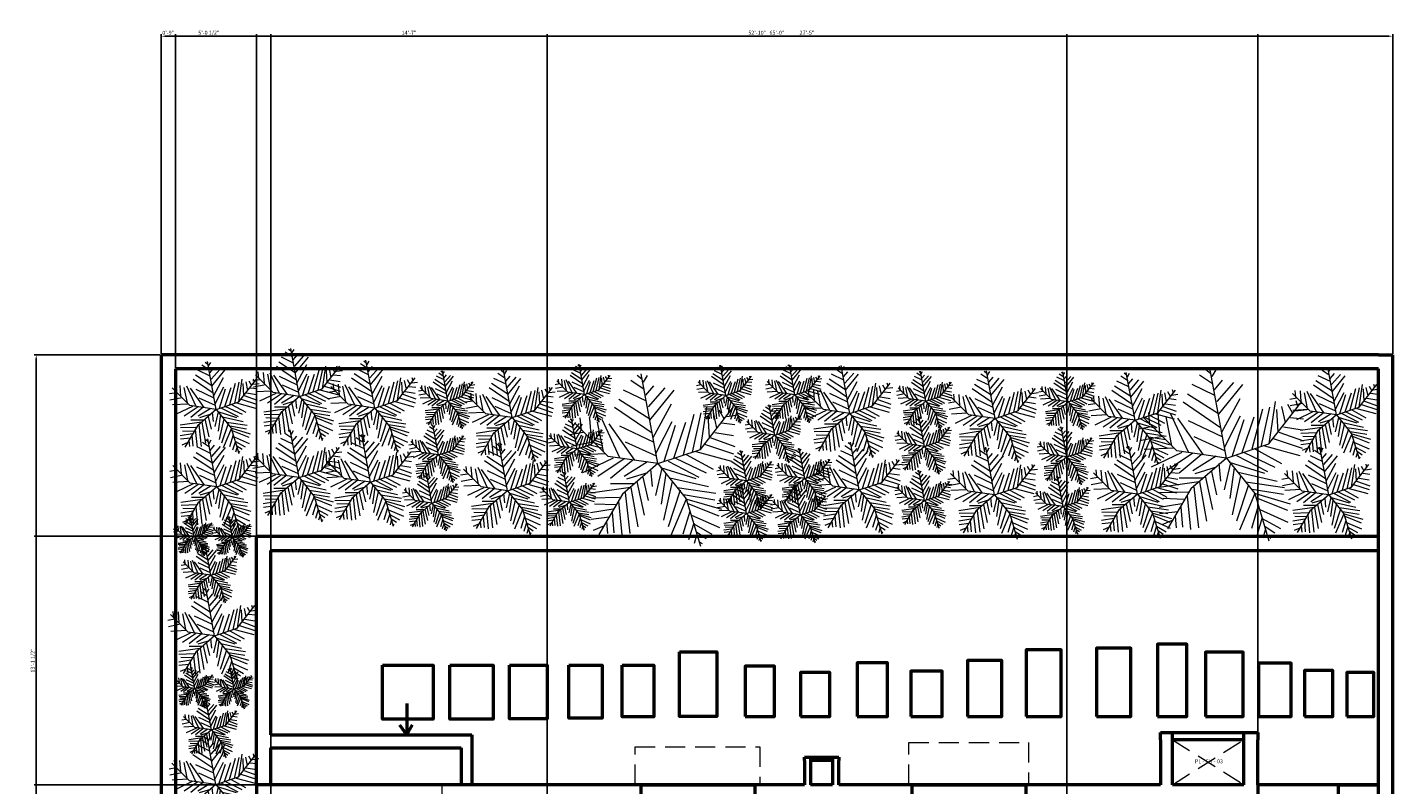
# Model space of a CAD drawing. Units: inches. Extents: x 5312 to 23584, y 2846 to 7447.
# Tile 4 of 12: x 8876 to 9740, y 3738 to 4217. Entities that reach past the tile are written whole.
import ezdxf

# ---------------------------------------------------------------- set-up
doc = ezdxf.new("R2010")
doc.units = ezdxf.units.IN
doc.linetypes.add('DASHED', pattern=[19.05, 12.7, -6.35])
for name, color, linetype, lineweight in [('A-ANNO-DIMS', 2, 'Continuous', 18), ('A-ANNO-TEXT', 3, 'Continuous', 18), ('A-FLOR-OVHD', 8, 'DASHED', 18), ('A-WALL', 7, 'Continuous', 50), ('L-PLNT', 82, 'Continuous', 13)]:
    doc.layers.add(name, color=color, linetype=linetype, lineweight=lineweight)
doc.styles.get("Standard").update_dxf_attribs({"font": 'arial.ttf'})
doc.dimstyles.new('ISO-25', dxfattribs={"dimtxt": 2.5, "dimasz": 2.5, "dimexe": 1.25, "dimexo": 0.625, "dimtad": 1, "dimlunit": 3, "dimtxsty": 'Standard', "dimcen": 2.5, "dimadec": 0, "dimazin": 0, "dimtfac": 1, "dimtmove": 0, "dimatfit": 3, "dimfxl": 1, "dimarcsym": 0})

# ---------------------------------------------------------------- blocks, each defined once
blk = doc.blocks.new('*U18')
for p, q in [((-8.737, 47.138), (-17.069, 52.711)), ((-10.186, 53.64), (-13.084, 55.962)), ((0, 0), (-10.5, 57)), ((-9.099, 51.782), (-6.563, 55.962)), ((-7.288, 39.707), (-21.778, 46.673)), ((-7.65, 43.423), (-2.578, 49.46)), ((-5.839, 35.992), (4.667, 48.067)), ((-5.114, 27.632), (10.463, 46.673)), ((-3.665, 19.273), (-27.574, 35.527)), ((-5.114, 28.097), (-24.676, 40.636)), ((-2.941, 16.486), (8.652, 37.85)), ((27, 9), (48, 36)), ((27.127, 9.056), (31.112, 35.992)), ((44.153, 36.456), (45.239, 32.741)), ((-48.585, 21.131), (-49.309, 29.026)), ((-43.513, 28.561), (-42.427, 15.558)), ((-38.442, 26.239), (-34.819, 7.663)), ((-35.544, 28.097), (-24.314, 3.947)), ((-1.129, 6.734), (9.014, 26.704)), ((10.101, 3.483), (17.708, 26.239)), ((16.259, 5.805), (23.142, 31.348)), ((22.055, 7.198), (27.489, 32.277)), ((31.836, 30.883), (32.561, 16.486)), ((35.096, 32.741), (37.27, 22.524)), ((38.719, 34.134), (41.979, 28.561)), ((43.791, 29.954), (51.036, 30.883)), ((-47.498, 19.737), (-55.83, 18.344)), ((-31.5, 4.5), (-52.5, 25.5)), ((-14.533, 2.09), (-30.834, 25.31)), ((-24.314, 23.917), (-2.941, 13.7)), ((3.942, 1.625), (11.187, 24.381)), ((36.183, 19.737), (48.137, 17.88)), ((40.53, 25.775), (48.862, 24.846)), ((-40.615, 13.7), (-55.105, 10.913)), ((-20.691, 13.7), (-1.129, 4.876)), ((0, 0), (27, 9)), ((29.662, 12.307), (48.137, 6.269)), ((33.285, 16.486), (48.862, 10.913)), ((-33.37, 6.269), (-52.207, 5.34)), ((-28.299, 3.483), (-47.86, -5.805)), ((-21.416, 3.018), (-38.079, -8.128)), ((0, 0), (-31.5, 4.5)), ((-15.982, 2.09), (-30.11, -9.521)), ((0, 0), (-22.5, -19.5)), ((-6.563, 1.161), (-21.416, -8.128)), ((0, 0), (18, -22.5)), ((6.478, 1.625), (26.04, -8.592)), ((11.187, 3.483), (30.749, -5.805)), ((18.07, 5.805), (35.096, -3.483)), ((24.229, 7.663), (46.688, 1.625)), ((-6.563, -5.805), (-19.967, -9.985)), ((-9.461, -8.592), (-6.201, -23.453)), ((-4.752, -3.483), (-3.665, -14.629)), ((2.493, -3.019), (-1.491, -20.202)), ((1.769, -2.555), (24.229, -9.521)), ((5.029, -6.27), (2.131, -25.775)), ((-17.431, -15.094), (-42.789, -18.809)), ((-15.257, -12.772), (-30.11, -12.772)), ((-17.069, -15.094), (-12.721, -40.172)), ((-13.446, -11.378), (-8.737, -32.741)), ((9.014, -11.378), (3.58, -35.992)), ((14.085, -16.951), (6.478, -40.172)), ((7.565, -9.056), (32.198, -14.629)), ((12.274, -15.094), (36.907, -18.809)), ((-24.314, -21.596), (-42.427, -22.06)), ((-26.849, -26.24), (-40.253, -25.775)), ((-22.5, -19.5), (-37.5, -45)), ((-25.038, -23.918), (-22.865, -45.281)), ((-20.691, -18.345), (-17.793, -44.352)), ((18.07, -22.524), (8.289, -45.745)), ((16.259, -19.738), (36.183, -22.989)), ((18, -22.5), (27, -52.5)), ((18.433, -22.524), (40.53, -29.026)), ((19.157, -25.311), (38.719, -33.206)), ((-28.299, -29.026), (-42.789, -31.348)), ((-30.834, -34.135), (-42.427, -35.528)), ((-29.023, -30.884), (-27.936, -43.887)), ((20.244, -30.419), (15.897, -44.816)), ((21.331, -32.741), (39.081, -40.636)), ((-34.457, -39.708), (-40.978, -42.494)), ((-32.646, -36.921), (-31.921, -44.352)), ((22.78, -37.85), (19.519, -48.532)), ((22.78, -38.314), (34.372, -44.816)), ((24.591, -45.745), (23.142, -50.854)), ((24.591, -43.423), (30.749, -47.603)), ((26.764, -49.925), (28.213, -50.854))]:
    blk.add_line(p, q)
blk = doc.blocks.new('*D46')
at = {"layer": 'A-ANNO-DIMS', "color": 0, "lineweight": -2, "transparency": 16777216}
for p, q in [((8960.57, 4010.46), (8960.57, 4212.68)), ((8963.07, 4211.43), (9737.82, 4211.43)), ((9740.32, 4010.46), (9740.32, 4212.68))]:
    blk.add_line(p, q, dxfattribs=at)
at = {"layer": 'A-ANNO-DIMS', "color": 0, "transparency": 16777216}
for points in [[(8963.07, 4211.85), (8963.07, 4211.01), (8960.57, 4211.43)], [(9737.82, 4211.85), (9737.82, 4211.01), (9740.32, 4211.43)]]:
    blk.add_solid(points, dxfattribs=at)
at = {"layer": 'DEFPOINTS', "color": 0, "transparency": 16777216}
for p in [(9740.32, 4211.43), (8960.57, 4009.84), (9740.32, 4009.84)]:
    blk.add_point(p, dxfattribs=at)
at = {"layer": 'A-ANNO-DIMS', "color": 0, "transparency": 16777216, "insert": (9350.45, 4213.33), "char_height": 2.5, "attachment_point": 5}
blk.add_mtext('65\'-0"', dxfattribs=at)
blk = doc.blocks.new('*D47')
at = {"layer": 'A-ANNO-DIMS', "color": 0, "lineweight": -2, "transparency": 16777216}
for p, q in [((8959.95, 4009.84), (8880.22, 4009.84)), ((8881.47, 4007.34), (8881.47, 2916.4)), ((8952.19, 2913.9), (8880.22, 2913.9))]:
    blk.add_line(p, q, dxfattribs=at)
at = {"layer": 'A-ANNO-DIMS', "color": 0, "transparency": 16777216}
for points in [[(8881.05, 4007.34), (8881.89, 4007.34), (8881.47, 4009.84)], [(8881.05, 2916.4), (8881.89, 2916.4), (8881.47, 2913.9)]]:
    blk.add_solid(points, dxfattribs=at)
at = {"layer": 'DEFPOINTS', "color": 0, "transparency": 16777216}
for p in [(8960.57, 4009.84), (8881.47, 2913.9), (8952.82, 2913.9)]:
    blk.add_point(p, dxfattribs=at)
at = {"layer": 'A-ANNO-DIMS', "color": 0, "transparency": 16777216, "insert": (8879.57, 3461.87), "char_height": 2.5, "attachment_point": 5, "rotation": 90}
blk.add_mtext('91\'-4"', dxfattribs=at)
blk = doc.blocks.new('*D48')
at = {"layer": 'A-ANNO-DIMS', "color": 0, "lineweight": -2, "transparency": 16777216}
for p, q in [((9021.01, 3738.27), (9021.01, 4212.68)), ((9023.51, 4211.43), (9652.51, 4211.43)), ((9655.01, 3738.27), (9655.01, 4212.68))]:
    blk.add_line(p, q, dxfattribs=at)
at = {"layer": 'A-ANNO-DIMS', "color": 0, "transparency": 16777216}
for points in [[(9023.51, 4211.85), (9023.51, 4211.01), (9021.01, 4211.43)], [(9652.51, 4211.85), (9652.51, 4211.01), (9655.01, 4211.43)]]:
    blk.add_solid(points, dxfattribs=at)
at = {"layer": 'DEFPOINTS', "color": 0, "transparency": 16777216}
for p in [(9655.01, 4211.43), (9021.01, 3737.65), (9655.01, 3737.65)]:
    blk.add_point(p, dxfattribs=at)
at = {"layer": 'A-ANNO-DIMS', "color": 0, "transparency": 16777216, "insert": (9338.01, 4213.33), "char_height": 2.5, "attachment_point": 5}
blk.add_mtext('52\'-10"', dxfattribs=at)
blk = doc.blocks.new('*D50')
at = {"layer": 'A-ANNO-DIMS', "color": 0, "lineweight": -2, "transparency": 16777216}
for p, q in [((8960.57, 4010.46), (8960.57, 4212.68)), ((8963.07, 4211.43), (9018.51, 4211.43)), ((9021.01, 3895.53), (9021.01, 4212.68))]:
    blk.add_line(p, q, dxfattribs=at)
at = {"layer": 'A-ANNO-DIMS', "color": 0, "transparency": 16777216}
for points in [[(8963.07, 4211.85), (8963.07, 4211.01), (8960.57, 4211.43)], [(9018.51, 4211.85), (9018.51, 4211.01), (9021.01, 4211.43)]]:
    blk.add_solid(points, dxfattribs=at)
at = {"layer": 'DEFPOINTS', "color": 0, "transparency": 16777216}
for p in [(9021.01, 4211.43), (8960.57, 4009.84), (9021.01, 3894.91)]:
    blk.add_point(p, dxfattribs=at)
at = {"layer": 'A-ANNO-DIMS', "color": 0, "transparency": 16777216, "insert": (8990.79, 4213.35), "char_height": 2.5, "attachment_point": 5}
blk.add_mtext('5\'-0 1/2"', dxfattribs=at)
blk = doc.blocks.new('*D51')
at = {"layer": 'A-ANNO-DIMS', "color": 0, "lineweight": -2, "transparency": 16777216}
for p, q in [((9020.38, 3894.91), (8880.22, 3894.91)), ((8881.47, 3892.41), (8881.47, 3740.15)), ((9020.38, 3737.65), (8880.22, 3737.65))]:
    blk.add_line(p, q, dxfattribs=at)
at = {"layer": 'A-ANNO-DIMS', "color": 0, "transparency": 16777216}
for points in [[(8881.05, 3892.41), (8881.89, 3892.41), (8881.47, 3894.91)], [(8881.05, 3740.15), (8881.89, 3740.15), (8881.47, 3737.65)]]:
    blk.add_solid(points, dxfattribs=at)
at = {"layer": 'DEFPOINTS', "color": 0, "transparency": 16777216}
for p in [(9021.01, 3894.91), (8881.47, 3737.65), (9021.01, 3737.65)]:
    blk.add_point(p, dxfattribs=at)
at = {"layer": 'A-ANNO-DIMS', "color": 0, "transparency": 16777216, "insert": (8879.55, 3816.28), "char_height": 2.5, "attachment_point": 5, "rotation": 90}
blk.add_mtext('13\'-1 1/2"', dxfattribs=at)
blk = doc.blocks.new('*D54')
at = {"layer": 'A-ANNO-DIMS', "color": 0, "lineweight": -2, "transparency": 16777216}
for p, q in [((9030.01, 3729.27), (9030.01, 4212.68)), ((9032.51, 4211.43), (9202.51, 4211.43)), ((9205.01, 3729.27), (9205.01, 4212.68))]:
    blk.add_line(p, q, dxfattribs=at)
at = {"layer": 'A-ANNO-DIMS', "color": 0, "transparency": 16777216}
for points in [[(9032.51, 4211.85), (9032.51, 4211.01), (9030.01, 4211.43)], [(9202.51, 4211.85), (9202.51, 4211.01), (9205.01, 4211.43)]]:
    blk.add_solid(points, dxfattribs=at)
at = {"layer": 'DEFPOINTS', "color": 0, "transparency": 16777216}
for p in [(9205.01, 4211.43), (9030.01, 3728.65), (9205.01, 3728.65)]:
    blk.add_point(p, dxfattribs=at)
at = {"layer": 'A-ANNO-DIMS', "color": 0, "transparency": 16777216, "insert": (9117.51, 4213.31), "char_height": 2.5, "attachment_point": 5}
blk.add_mtext('14\'-7"', dxfattribs=at)
blk = doc.blocks.new('*D55')
at = {"layer": 'A-ANNO-DIMS', "color": 0, "lineweight": -2, "transparency": 16777216}
for p, q in [((9205.01, 3729.27), (9205.01, 4212.68)), ((9207.51, 4211.43), (9531.51, 4211.43)), ((9534.01, 3705.2), (9534.01, 4212.68))]:
    blk.add_line(p, q, dxfattribs=at)
at = {"layer": 'A-ANNO-DIMS', "color": 0, "transparency": 16777216}
for points in [[(9207.51, 4211.85), (9207.51, 4211.01), (9205.01, 4211.43)], [(9531.51, 4211.85), (9531.51, 4211.01), (9534.01, 4211.43)]]:
    blk.add_solid(points, dxfattribs=at)
at = {"layer": 'DEFPOINTS', "color": 0, "transparency": 16777216}
for p in [(9534.01, 4211.43), (9205.01, 3728.65), (9534.01, 3704.57)]:
    blk.add_point(p, dxfattribs=at)
at = {"layer": 'A-ANNO-DIMS', "color": 0, "transparency": 16777216, "insert": (9369.51, 4213.33), "char_height": 2.5, "attachment_point": 5}
blk.add_mtext('27\'-5"', dxfattribs=at)
blk = doc.blocks.new('*D57')
at = {"layer": 'A-ANNO-DIMS', "color": 0, "lineweight": -2, "transparency": 16777216}
for p, q in [((8960.57, 4010.46), (8960.57, 4212.68)), ((8963.07, 4211.43), (8967.07, 4211.43)), ((8969.57, 4001.46), (8969.57, 4212.68))]:
    blk.add_line(p, q, dxfattribs=at)
at = {"layer": 'A-ANNO-DIMS', "color": 0, "transparency": 16777216}
for points in [[(8963.07, 4211.85), (8963.07, 4211.01), (8960.57, 4211.43)], [(8967.07, 4211.85), (8967.07, 4211.01), (8969.57, 4211.43)]]:
    blk.add_solid(points, dxfattribs=at)
at = {"layer": 'DEFPOINTS', "color": 0, "transparency": 16777216}
for p in [(8969.57, 4211.43), (8960.57, 4009.84), (8969.57, 4000.84)]:
    blk.add_point(p, dxfattribs=at)
at = {"layer": 'A-ANNO-DIMS', "color": 0, "transparency": 16777216, "insert": (8965.07, 4213.33), "char_height": 2.5, "attachment_point": 5}
blk.add_mtext('0\'-9"', dxfattribs=at)

msp = doc.modelspace()

# ---------------------------------------------------------------- linework, layer by layer
at = {"layer": 'A-FLOR-OVHD'}
for p, q in [((9260.644, 3737.646), (9260.644, 3761.587)), ((9260.644, 3761.587), (9339.603, 3761.587)), ((9339.603, 3761.587), (9339.603, 3737.646)), ((9433.958, 3737.646), (9433.958, 3764.447)), ((9433.958, 3764.447), (9509.769, 3764.447)), ((9509.769, 3764.447), (9509.769, 3737.646)), ((9600.965, 3765.999), (9600.965, 3765.999)), ((9600.965, 3765.999), (9646.009, 3737.646)), ((9600.965, 3737.646), (9646.009, 3765.999)), ((9138.223, 3737.646), (9138.223, 3378.646))]:
    msp.add_line(p, q, dxfattribs=at)
at = {"layer": 'A-WALL'}
for p, q in [((9021.009, 4009.837), (8960.573, 4009.837)), ((8960.573, 4009.837), (8960.573, 3030.646)), ((9731.323, 4009.837), (9021.009, 4009.837)), ((9731.323, 4009.837), (9740.323, 4009.837)), ((9740.323, 3061.779), (9740.323, 4009.837)), ((9731.323, 4000.837), (8969.573, 4000.837)), ((8969.573, 4000.837), (8969.573, 3030.646)), ((9731.323, 3061.779), (9731.323, 4000.837)), ((9021.009, 3769.262), (9021.009, 3894.906)), ((9021.009, 3894.906), (9731.323, 3894.906)), ((9030.009, 3885.906), (9731.323, 3885.906)), ((9030.009, 3769.262), (9030.009, 3885.906)), ((9116.057, 3788.994), (9116.057, 3769.262)), ((9021.009, 3737.646), (9021.009, 3769.262)), ((9030.009, 3769.262), (9157.207, 3769.262)), ((9116.057, 3769.262), (9111.665, 3775.357)), ((9116.057, 3769.262), (9119.732, 3775.533)), ((9116.057, 3769.262), (9116.057, 3769.262)), ((9157.207, 3769.262), (9157.207, 3737.646)), ((9593.222, 3765.999), (9593.222, 3770.585)), ((9593.222, 3770.585), (9655.009, 3770.585)), ((9600.965, 3737.646), (9600.965, 3770.585)), ((9646.009, 3737.646), (9646.009, 3770.585)), ((9655.009, 3770.585), (9655.009, 3765.999)), ((9030.009, 3761.073), (9150.611, 3761.073)), ((9030.009, 3737.646), (9030.009, 3761.073)), ((9150.611, 3761.073), (9150.611, 3737.646)), ((9593.222, 3765.999), (9593.222, 3737.646)), ((9646.009, 3765.999), (9600.965, 3765.999)), ((9655.009, 3737.646), (9655.009, 3765.999)), ((9367.943, 3752.998), (9367.943, 3755.169)), ((9367.943, 3755.169), (9389.615, 3755.169)), ((9367.943, 3752.998), (9367.943, 3737.646)), ((9371.678, 3755.169), (9371.678, 3737.646)), ((9385.647, 3752.998), (9371.678, 3752.998)), ((9385.647, 3755.169), (9385.647, 3737.646)), ((9389.615, 3755.169), (9389.615, 3752.998)), ((9389.615, 3737.646), (9389.615, 3752.998)), ((9021.009, 3737.646), (9021.009, 3030.646)), ((9367.943, 3737.646), (9021.009, 3737.646)), ((9264.453, 3728.646), (9264.453, 3737.646)), ((9264.453, 3737.646), (9336.453, 3737.646)), ((9336.453, 3737.646), (9336.453, 3728.646)), ((9385.647, 3737.646), (9371.678, 3737.646)), ((9593.222, 3737.646), (9389.615, 3737.646)), ((9436.116, 3728.646), (9436.116, 3737.646)), ((9436.116, 3737.646), (9508.116, 3737.646)), ((9508.116, 3737.646), (9508.116, 3728.646)), ((9646.009, 3737.646), (9600.965, 3737.646)), ((9731.323, 3737.646), (9655.009, 3737.646)), ((9655.009, 3737.646), (9655.009, 3554.646)), ((9705.72, 3737.646), (9705.72, 3650.559)), ((9705.72, 3737.646), (9731.323, 3737.646))]:
    msp.add_line(p, q, dxfattribs=at)
for points in [[(9288.745, 3821.65), (9312.403, 3821.65), (9312.403, 3780.72), (9288.745, 3780.72)], [(9508.355, 3780.72), (9530.463, 3780.72), (9530.463, 3823.042), (9508.355, 3823.042)], [(9552.791, 3780.72), (9574.515, 3780.72), (9574.515, 3824.124), (9552.791, 3824.124)], [(9591.341, 3780.72), (9610.049, 3780.72), (9610.049, 3826.673), (9591.341, 3826.673)], [(9621.859, 3780.72), (9645.675, 3780.72), (9645.675, 3821.61), (9621.859, 3821.61)], [(9100.64, 3813.302), (9132.752, 3813.302), (9132.752, 3779.081), (9100.64, 3779.081)], [(9143.345, 3813.302), (9170.737, 3813.302), (9170.737, 3779.203), (9143.345, 3779.203)], [(9181.077, 3813.302), (9205.071, 3813.302), (9205.071, 3779.385), (9181.077, 3779.385)], [(9218.765, 3813.302), (9239.757, 3813.302), (9239.757, 3779.802), (9218.765, 3779.802)], [(9252.47, 3813.302), (9272.606, 3813.302), (9272.606, 3780.515), (9252.47, 3780.515)], [(9330.272, 3780.72), (9348.871, 3780.72), (9348.871, 3812.622), (9330.272, 3812.622)], [(9401.17, 3780.72), (9420.378, 3780.72), (9420.378, 3814.818), (9401.17, 3814.818)], [(9471.206, 3780.72), (9492.776, 3780.72), (9492.776, 3816.212), (9471.206, 3816.212)], [(9655.264, 3780.72), (9675.985, 3780.72), (9675.985, 3814.641), (9655.264, 3814.641)], [(9365.391, 3780.72), (9383.862, 3780.72), (9383.862, 3808.56), (9365.391, 3808.56)], [(9435.332, 3780.72), (9454.995, 3780.72), (9454.995, 3809.417), (9435.332, 3809.417)], [(9684.579, 3780.72), (9702.434, 3780.72), (9702.434, 3809.983), (9684.579, 3809.983)], [(9711.281, 3780.72), (9728.352, 3780.72), (9728.352, 3808.708), (9711.281, 3808.708)]]:
    msp.add_lwpolyline(points, close=True, dxfattribs=at)

# ---------------------------------------------------------------- block references
at = {"layer": 'L-PLNT'}
for p, xscale, yscale, zscale in [((9048.234, 3983.472), 0.5312656759052281, 0.5312656759052281, 0.5312656759052281), ((8995.434, 3975.22), 0.5312656759052281, 0.5312656759052281, 0.5312656759052281), ((9095.816, 3976.073), 0.5312656759052281, 0.5312656759052281, 0.5312656759052281), ((9228.713, 3984.679), 0.3351400291328743, 0.3351400291328743, 0.3351400291328743), ((9318.192, 3984.08), 0.3351400291328743, 0.3351400291328743, 0.3351400291328743), ((9361.844, 3984.393), 0.3351400291328743, 0.3351400291328743, 0.3351400291328743), ((9396.62, 3972.675), 0.5312656759052281, 0.5312656759052281, 0.5312656759052281), ((9142.137, 3980.519), 0.3351400291328743, 0.3351400291328743, 0.3351400291328743), ((9182.838, 3970.014), 0.5312656759052281, 0.5312656759052281, 0.5312656759052281), ((9275.047, 3940.917), 0.996741466224922, 0.996741466224922, 0.996741466224922), ((9444.793, 3980.374), 0.3351400291328743, 0.3351400291328743, 0.3351400291328743), ((9488.676, 3969.414), 0.5312656759052281, 0.5312656759052281, 0.5312656759052281), ((9534.93, 3979.913), 0.3351400291328743, 0.3351400291328743, 0.3351400291328743), ((9577.202, 3968.342), 0.5312656759052281, 0.5312656759052281, 0.5312656759052281), ((9635.045, 3944.417), 0.996741466224922, 0.996741466224922, 0.996741466224922), ((9704.762, 3971.752), 0.5312656759052281, 0.5312656759052281, 0.5312656759052281), ((9349.027, 3958.987), 0.3351400291328743, 0.3351400291328743, 0.3351400291328743), ((9223.926, 3950.238), 0.3351400291328743, 0.3351400291328743, 0.3351400291328743), ((9443.877, 3951.808), 0.3351400291328743, 0.3351400291328743, 0.3351400291328743), ((9047.899, 3932.02), 0.5312656759052281, 0.5312656759052281, 0.5312656759052281), ((9136.203, 3946.427), 0.3351400291328743, 0.3351400291328743, 0.3351400291328743), ((9533.958, 3945.151), 0.3351400291328743, 0.3351400291328743, 0.3351400291328743), ((8995.769, 3926.195), 0.5312656759052281, 0.5312656759052281, 0.5312656759052281), ((9093.172, 3929.108), 0.5312656759052281, 0.5312656759052281, 0.5312656759052281), ((9179.856, 3923.73), 0.5312656759052281, 0.5312656759052281, 0.5312656759052281), ((9402.58, 3924.234), 0.5312656759052281, 0.5312656759052281, 0.5312656759052281), ((9488.302, 3921.049), 0.5312656759052281, 0.5312656759052281, 0.5312656759052281), ((9578.734, 3921.564), 0.5312656759052281, 0.5312656759052281, 0.5312656759052281), ((9699.811, 3921.107), 0.5312656759052281, 0.5312656759052281, 0.5312656759052281), ((9331.146, 3930.061), 0.3351400291328743, 0.3351400291328743, 0.3351400291328743), ((9368.046, 3931.515), 0.3351400291328743, 0.3351400291328743, 0.3351400291328743), ((9132.036, 3915.936), 0.3351400291328743, 0.3351400291328743, 0.3351400291328743), ((9219.139, 3916.435), 0.3351400291328743, 0.3351400291328743, 0.3351400291328743), ((9443.882, 3917.534), 0.3351400291328743, 0.3351400291328743, 0.3351400291328743), ((9331.249, 3909.207), 0.3351400291328743, 0.3351400291328743, 0.3351400291328743), ((9365.358, 3908.381), 0.3351400291328743, 0.3351400291328743, 0.3351400291328743), ((9531.659, 3913.782), 0.3351400291328743, 0.3351400291328743, 0.3351400291328743), ((8981.449, 3894.836), 0.2364091890538949, 0.2364091890538949, 0.2364091890538949), ((9005.808, 3894.009), 0.2364091890538949, 0.2364091890538949, 0.2364091890538949), ((8992.023, 3870.262), 0.3351400291328743, 0.3351400291328743, 0.3351400291328743), ((8994.407, 3831.877), 0.5312656759052281, 0.5312656759052281, 0.5312656759052281), ((8981.929, 3798.57), 0.2364091890538949, 0.2364091890538949, 0.2364091890538949), ((9006.815, 3798.083), 0.2364091890538949, 0.2364091890538949, 0.2364091890538949), ((8992.379, 3772.342), 0.3351400291328743, 0.3351400291328743, 0.3351400291328743), ((8995.269, 3737.769), 0.5312656759052281, 0.5312656759052281, 0.5312656759052281)]:
    msp.add_blockref('*U18', p, dxfattribs=dict(at, xscale=xscale, yscale=yscale, zscale=zscale))

# ---------------------------------------------------------------- texts
at = {"layer": 'A-ANNO-TEXT', "insert": (9615.092, 3753.693), "char_height": 2.5, "attachment_point": 1}
msp.add_mtext_dynamic_manual_height_columns('PL - SH - 03', width=31.65843, gutter_width=12.5, heights=[0], dxfattribs=at)

# ---------------------------------------------------------------- dimensions: what is measured, and where the dimension line sits
at = {"layer": 'A-ANNO-DIMS'}
for base, p1, p2, picture, middle in [((9021.009, 4211.429), (8960.573, 4009.837), (9021.009, 3894.906), '*D50', (8990.791, 4213.346)), ((9740.3234, 4211.4289), (8960.5729, 4009.8369), (9740.3234, 4009.8369), '*D46', (9350.4481, 4213.3303)), ((8969.573, 4211.429), (8960.573, 4009.837), (8969.573, 4000.837), '*D57', (8965.073, 4213.33)), ((9655.009, 4211.429), (9021.009, 3737.646), (9655.009, 3737.646), '*D48', (9338.009, 4213.33)), ((9205.009, 4211.429), (9030.009, 3728.646), (9205.009, 3728.646), '*D54', (9117.509, 4213.309)), ((9534.009, 4211.429), (9205.009, 3728.646), (9534.009, 3704.571), '*D55', (9369.509, 4213.33))]:
    dim = msp.add_linear_dim(base=base, p1=p1, p2=p2, dimstyle='ISO-25', override={"dimdec": 1, "dimlfac": 1, "dimrnd": 0, "dimzin": 1, "dimdsep": 46, "dimlunit": 4, "dimfrac": 2}, dxfattribs=at)
    dim.commit()
    dim.dimension.update_dxf_attribs({"geometry": picture, "text_midpoint": middle})
for base, p1, p2, picture, middle in [((8881.47, 2913.9), (8960.573, 4009.837), (8952.82, 2913.9), '*D47', (8879.569, 3461.869)), ((8881.47, 3737.646), (9021.009, 3894.906), (9021.009, 3737.646), '*D51', (8879.552, 3816.276))]:
    dim = msp.add_linear_dim(base=base, p1=p1, p2=p2, angle=90, dimstyle='ISO-25', override={"dimdec": 1, "dimlfac": 1, "dimrnd": 0, "dimzin": 1, "dimdsep": 46, "dimlunit": 4, "dimfrac": 2}, dxfattribs=at)
    dim.commit()
    dim.dimension.update_dxf_attribs({"geometry": picture, "text_midpoint": middle})

doc.saveas('drawing.dxf')
